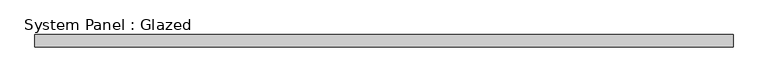
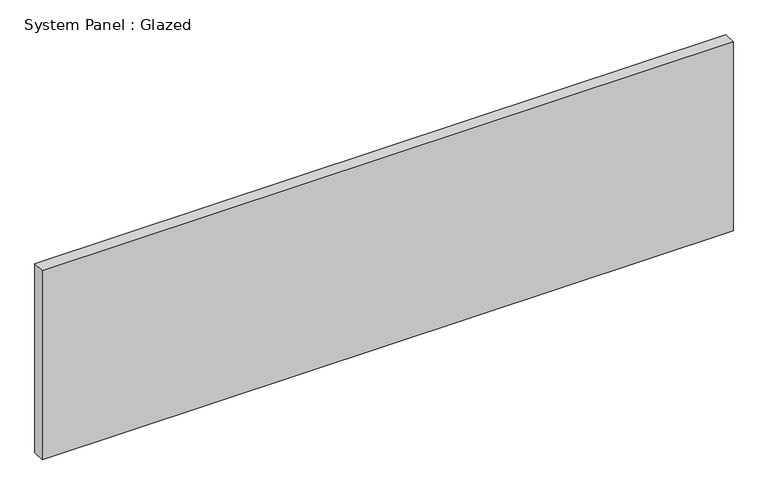
"""IFC4 building model written with IfcOpenShell, lengths in millimetres: plate geometry, System Panel : Glazed."""

from ifc_helpers import new_model, si_unit, origin, origin_with_axes, place, context, project, spatial, polyline, outline, extrude, source, transform, mapped, element, save


def system_panel_glazed_03bb9a0f(model_context):
    return source(origin(), model_context, "Body", "SweptSolid", [
        extrude(outline(polyline([(714.375, 19.05), (-714.375, 19.05), (-714.375, 44.45), (714.375, 44.45), (714.375, 19.05)])), origin_with_axes(), (0.0, 0.0, 1.0), 412.75),
    ])


if __name__ == "__main__":
    model = new_model("IFC4")
    model_context = context("Model", 3, world=origin())
    ifc_project = project(units=[si_unit("LENGTHUNIT", "METRE", prefix="MILLI")], contexts=[model_context])
    site = spatial("IfcSite", under=ifc_project)
    building = spatial("IfcBuilding", under=site)
    placement = place(None, origin())
    system_panel_glazed_shape = system_panel_glazed_03bb9a0f(model_context)
    element("IfcPlate", 1, ObjectType="System Panel : Glazed", at=placement, inside=building, context=model_context, shape_type="MappedRepresentation", body=[
        mapped(system_panel_glazed_shape, transform((0.0, 0.0, 0.0), x_axis=(1.0, 0.0, 0.0), y_axis=(0.0, 1.0, 0.0), z_axis=(0.0, 0.0, 1.0))),
    ])
    save(model, "model.ifc")

# Revit data of these elements
# Type "System Panel : Glazed"
#   Construction Type Id = "GSP4R"
#   Analytic Construction = "1/8 in Pilkington single glazing"
#   Visual Light Transmittance = 0.9
#   Solar Heat Gain Coefficient = 0.86
#   Heat Transfer Coefficient (U) = 1.18115 BTU/(h·ft²·°F)
#   Define Thermal Properties by = 1
# Element 1 (IfcPlate, "System Panel : Glazed")
#   Materials on its faces: "Glass"
# Materials
#   "Glass": class "Glass", colour RGB 0 128 192, transparency 0.75, Description = "Soda Lime Glass", Cost = 0
